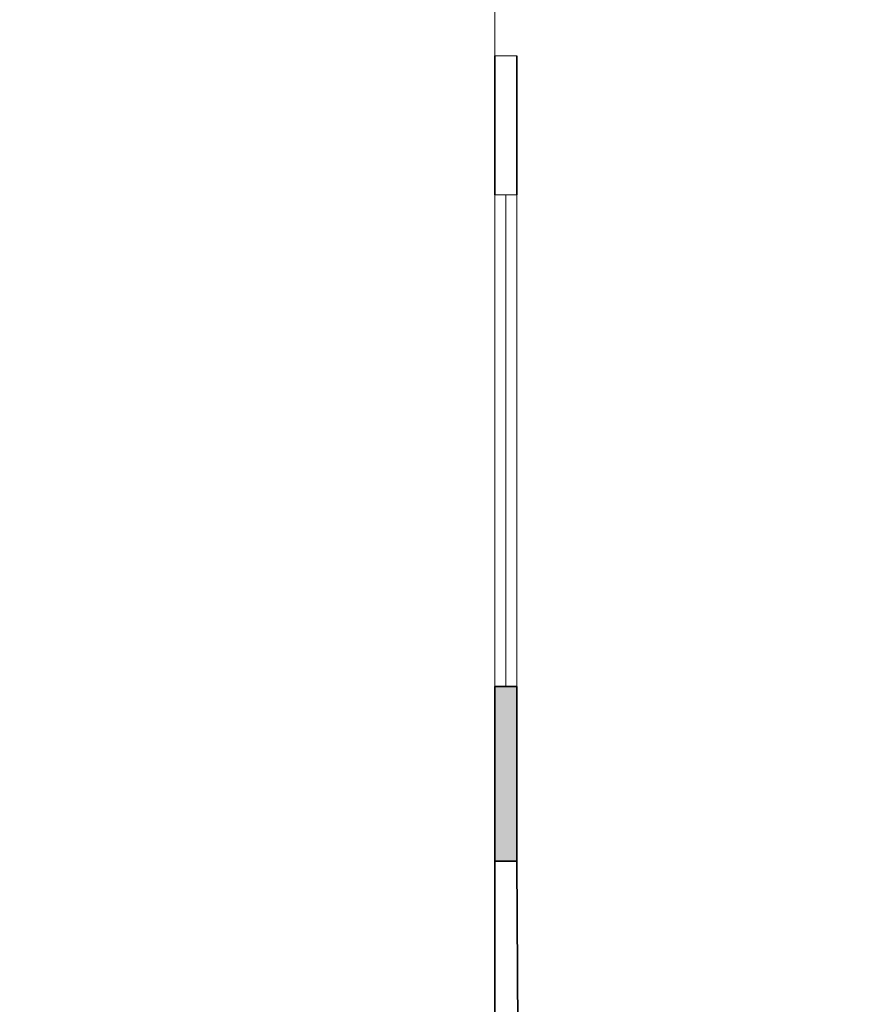
# Model space of a CAD drawing. Units: inches. Extents: x 1002 to 1561, y 1016 to 1994.
# Tile 3 of 8: x 1166 to 1282, y 1149 to 1283. Entities that reach past the tile are written whole.
import ezdxf

# ---------------------------------------------------------------- set-up
doc = ezdxf.new("R2010")
doc.units = ezdxf.units.IN
doc.header["$MEASUREMENT"] = 0
doc.layers.add('A-DOOR', color=30, linetype='Continuous', lineweight=18, true_color=0xf8991e)
doc.layers.add('A-GLAZ', color=217, linetype='Continuous', lineweight=18, true_color=0x93278f)
doc.layers.add('A-WALL', color=7, linetype='Continuous', lineweight=35)
doc.layers.add('A-WALL-PATT', color=7, linetype='Continuous', lineweight=13)

msp = doc.modelspace()

# ---------------------------------------------------------------- hatches: boundary and pattern name
at = {"layer": 'A-WALL-PATT'}
h = msp.add_hatch(color=256, dxfattribs=at)
h.dxf.hatch_style = 1
h.paths.add_polyline_path([(1206.434, 1924.784), (1203.434, 1924.784), (1203.434, 1898.155), (1206.434, 1898.155)])
h.paths.add_polyline_path([(1326.434, 1925.745), (1323.434, 1925.745), (1323.434, 1900.458), (1326.434, 1900.458)])
h.paths.add_polyline_path([(1290.434, 1840.51), (1287.434, 1840.51), (1287.434, 1837.51), (1287.434, 1823.284), (1290.434, 1823.284)])
h.paths.add_polyline_path([(1287.434, 1840.51), (1285.684, 1840.51), (1285.684, 1837.51), (1287.434, 1837.51)])
h.paths.add_polyline_path([(1233.434, 1840.51), (1230.434, 1840.51), (1230.434, 1823.284), (1233.434, 1823.284)])
h.paths.add_polyline_path([(1235.119, 1840.51), (1233.434, 1840.51), (1233.434, 1837.51), (1235.119, 1837.51)])
h.paths.add_polyline_path([(1050.434, 1837.51), (1050.434, 1840.51), (1046.434, 1840.51), (1046.434, 1814.619), (1050.434, 1814.619)])
h.paths.add_polyline_path([(1050.434, 1682.088), (1046.434, 1682.088), (1046.434, 1648.51), (1046.434, 1645.51), (1050.434, 1645.51), (1050.434, 1648.51)])
h.paths.add_polyline_path([(1233.434, 1648.51), (1211.636, 1648.51), (1211.636, 1645.51), (1233.434, 1645.51)])
h.paths.add_polyline_path([(1307.549, 1648.51), (1287.434, 1648.51), (1287.434, 1645.51), (1307.549, 1645.51)])
h.paths.add_polyline_path([(1516.434, 1927.595), (1512.434, 1927.595), (1512.434, 1896.846), (1516.434, 1896.846)])
h.paths.add_polyline_path([(1516.434, 1840.51), (1512.434, 1840.51), (1512.434, 1816.31), (1516.434, 1816.31)])
h.paths.add_polyline_path([(1516.434, 1686.827), (1512.434, 1686.827), (1512.434, 1645.51), (1516.434, 1645.51)])
h.paths.add_polyline_path([(1472.434, 1321.51), (1469.434, 1321.51), (1469.434, 1306.51), (1472.434, 1306.51)])
h.paths.add_polyline_path([(1295.733, 1141.51), (1281.793, 1141.51), (1281.793, 1137.51), (1295.733, 1137.51)])
h.paths.add_polyline_path([(1239.434, 1321.51), (1230.434, 1321.51), (1230.434, 1318.51), (1239.434, 1318.51)])
h.paths.add_polyline_path([(1290.434, 1332.122), (1287.434, 1332.122), (1287.434, 1318.51), (1290.434, 1318.51)])
h.paths.add_polyline_path([(1311.434, 1480.51), (1287.434, 1480.51), (1287.434, 1477.51), (1311.434, 1477.51)])
h.paths.add_polyline_path([(1050.434, 1480.51), (1046.434, 1480.51), (1046.434, 1468.51), (1050.434, 1468.51)])
h.paths.add_polyline_path([(1050.434, 1321.51), (1046.434, 1321.51), (1046.434, 1309.51), (1050.434, 1309.51)])
h.paths.add_polyline_path([(1233.434, 1192.382), (1230.434, 1192.382), (1230.434, 1168.702), (1233.434, 1168.702)])
h.paths.add_polyline_path([(1050.434, 1137.51), (1046.434, 1137.51), (1046.434, 1119.51), (1050.434, 1119.51)])
h.paths.add_polyline_path([(1472.434, 1153.51), (1469.434, 1153.51), (1469.434, 1141.51), (1472.434, 1141.51)])
h.paths.add_polyline_path([(1472.434, 1141.51), (1469.434, 1141.51), (1469.434, 1137.51), (1472.434, 1137.51)])

# ---------------------------------------------------------------- linework, layer by layer
at = {"layer": 'A-DOOR'}
for q in [(1230.434, 1318.51), (1233.434, 1277.919)]:
    msp.add_line((1230.434, 1277.919), q, dxfattribs=at)
at = {"layer": 'A-GLAZ'}
for p, q in [((1233.434, 1259.072), (1230.434, 1259.072)), ((1230.434, 1259.072), (1230.434, 1192.382)), ((1233.434, 1259.072), (1231.941, 1259.072)), ((1231.941, 1259.072), (1231.941, 1192.382)), ((1233.434, 1192.382), (1233.434, 1259.072)), ((1230.434, 1192.382), (1233.434, 1192.382))]:
    msp.add_line(p, q, dxfattribs=at)
at = {"layer": 'A-WALL'}
for p, q in [((1230.434, 1259.072), (1230.434, 1277.919)), ((1233.434, 1259.072), (1233.434, 1277.919)), ((1230.434, 1168.702), (1230.434, 1192.382)), ((1230.434, 1192.382), (1233.434, 1192.382)), ((1233.434, 1168.702), (1233.434, 1192.382)), ((1233.434, 1168.702), (1230.434, 1168.702)), ((1230.434, 1168.702), (1230.434, 1121.51)), ((1233.434, 1168.702), (1233.773, 1119.51))]:
    msp.add_line(p, q, dxfattribs=at)

doc.saveas('drawing.dxf')
